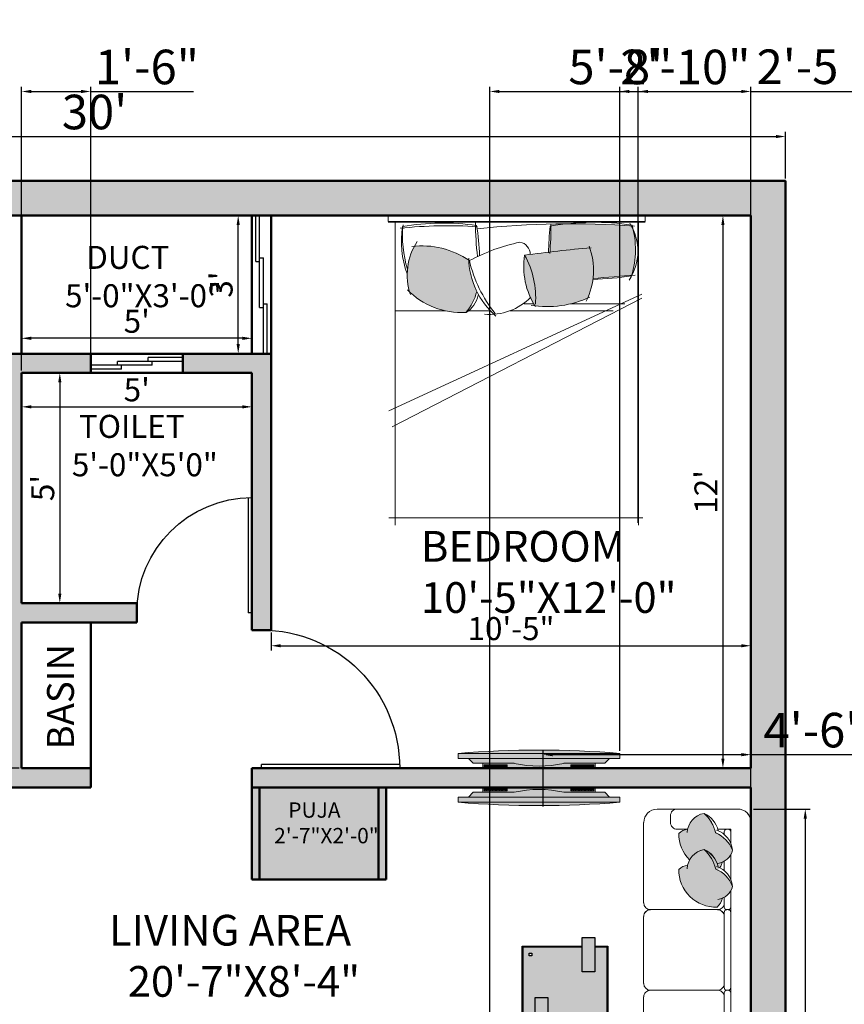
# Model space of a CAD drawing. Units: inches. Extents: x 3274 to 5176, y 1085 to 2172.
# Tile 14 of 16: x 4518 to 4733, y 1319 to 1575. Entities that reach past the tile are written whole.
import ezdxf

# ---------------------------------------------------------------- set-up
doc = ezdxf.new("R2010")
doc.units = ezdxf.units.IN
for name, color, linetype, lineweight in [('0.10', 252, 'Continuous', 9), ('A-ANNO-DIMS', 2, 'Continuous', 18), ('A-AREA-IDEN', 3, 'Continuous', 25), ('A-DOOR', 4, 'Continuous', 25), ('A-EQPM', 8, 'Continuous', 18), ('A-FLOR-PATT', 252, 'Continuous', 13), ('A-FURN', 8, 'Continuous', 18), ('A-GLAZ', 5, 'Continuous', 25), ('A-WALL', 7, 'Continuous', 50), ('A-WALL-PATT', 8, 'Continuous', 13), ('moveis', 254, 'Continuous', 5), ('parede', 7, 'Continuous', 30)]:
    doc.layers.add(name, color=color, linetype=linetype, lineweight=lineweight)
doc.layers.add('MOBIL', color=7, linetype='Continuous')
doc.styles.get("Standard").update_dxf_attribs({"font": 'arial.ttf'})
doc.dimstyles.new('ISO-25', dxfattribs={"dimtxt": 9, "dimasz": 2.5, "dimexe": 1.25, "dimexo": 0.625, "dimtad": 1, "dimdec": 1, "dimlunit": 3, "dimtxsty": 'Standard', "dimcen": 2.5, "dimclrd": 4, "dimclre": 4, "dimclrt": 1, "dimadec": 0, "dimazin": 0, "dimtfac": 1, "dimtdec": 1, "dimtmove": 0, "dimatfit": 3, "dimfxl": 1, "dimarcsym": 0})

# ---------------------------------------------------------------- blocks, each defined once
blk = doc.blocks.new('2')
for p, q in [((0, 30), (0, 0)), ((1, 30), (1, 0)), ((0, 0), (1, 0))]:
    blk.add_line(p, q)
blk.add_arc((0, 0), 30, 0, 90)
blk = doc.blocks.new('1')
for p, q in [((0, 36), (0, 0)), ((1, 36), (1, 0)), ((0, 0), (1, 0))]:
    blk.add_line(p, q)
blk.add_arc((0, 0), 36, 0, 90)
blk = doc.blocks.new('*D6')
at = {"layer": 'A-ANNO-DIMS', "color": 0, "lineweight": -2, "transparency": 16777216}
for p, q in [((4357.19, 1533.98), (4357.19, 1546.17)), ((4359.69, 1544.92), (4714.69, 1544.92)), ((4717.19, 1533.98), (4717.19, 1546.17))]:
    blk.add_line(p, q, dxfattribs=at)
at = {"layer": 'A-ANNO-DIMS', "color": 0, "transparency": 16777216}
for points in [[(4359.69, 1545.33), (4359.69, 1544.5), (4357.19, 1544.92)], [(4714.69, 1545.33), (4714.69, 1544.5), (4717.19, 1544.92)]]:
    blk.add_solid(points, dxfattribs=at)
at = {"layer": 'Defpoints', "color": 0, "transparency": 16777216}
for p in [(4717.19, 1544.92), (4357.19, 1533.35), (4717.19, 1533.35)]:
    blk.add_point(p, dxfattribs=at)
at = {"layer": 'A-ANNO-DIMS', "color": 0, "transparency": 16777216, "insert": (4537.19, 1550.14), "char_height": 9, "attachment_point": 5}
blk.add_mtext("30'", dxfattribs=at)
blk = doc.blocks.new('camita')
at = {"layer": '0.10'}
for p, q in [((-0.85, -0.045), (0.85, -0.045)), ((-0.805, -0.045), (-0.805, -2.0485)), ((0.805, -0.045), (0.805, -2.0485)), ((-0.8271, -0.521), (0.8464, -1.2932)), ((-0.8271, -0.5476), (0.8236, -1.3992)), ((-0.7161, -0.585), (-0.3554, -0.585)), ((-0.1136, -0.585), (-0.0485, -0.585)), ((-0.638, -0.63), (0.0434, -0.63)), ((0.1749, -0.63), (0.3179, -0.63)), ((0.4739, -0.63), (0.805, -0.63)), ((-0.8354, -2), (0.8464, -2))]:
    blk.add_line(p, q, dxfattribs=at)
blk.add_lwpolyline([(-0.85, -0.0405), (0.85, -0.0405), (0.85, 0), (-0.85, 0)], close=True, dxfattribs=at)
for centre, radius, start, end in [((-0.4574, -0.2364), 0.3443, 147.50996, 213.83359), ((-0.1997, -0.2266), 0.5864, 163.92635, 197.14087), ((-0.3639, -5.8457), 5.7909, 83.80731, 94.12107), ((-0.5104, -1.7232), 1.6781, 80.12554, 98.66187), ((2.3534, -0.0532), 2.5803, 180.10628, 184.38541), ((-1.4396, -0.0609), 1.7117, 352.92911, 0.39592), ((0.4863, -1.6286), 1.5781, 80.16015, 98.05996), ((0.0294, -0.1377), 0.7262, 342.58415, 6.00484), ((-1.5443, -0.2452), 1.3333, 359.93941, 7.55329), ((1.5815, -0.2893), 1.3353, 170.38021, 178.99138), ((0.4524, -3.0675), 2.9996, 83.90257, 93.67595), ((0.1326, -0.1696), 0.6307, 339.92303, 8.74334), ((-0.007, -0.258), 0.0828, 100.01798, 179.73597), ((-0.2931, -1.4378), 1.2903, 61.97485, 77.84351), ((0.3203, -0.3944), 0.4043, 341.45245, 33.45121), ((-0.0543, -0.3633), 0.4542, 159.30257, 206.50263), ((-1.3301, -9.6748), 9.4985, 82.27078, 84.93989), ((0.6265, -0.7518), 0.5508, 82.96906, 124.67388), ((0.4585, -0.5454), 0.5842, 151.04555, 184.14969), ((-0.5341, -0.3393), 0.4875, 327.26442, 9.0473), ((-0.1986, -0.2742), 0.5159, 310.73945, 359.05759), ((-0.5673, -0.0868), 0.9057, 321.69527, 346.46261), ((-1.8672, -14.986), 14.6323, 84.65974, 85.75157), ((-0.4598, 1.4861), 1.9092, 260.95299, 268.65169), ((0.5707, -0.4317), 0.3145, 192.93877, 221.96363), ((0.3612, -0.133), 0.5096, 267.25889, 315.29965), ((-0.2002, 0.064), 0.6673, 244.78094, 279.06058), ((0.179, -0.272), 0.3828, 224.52836, 275.22287), ((0.4384, -0.4834), 0.1898, 193.68485, 236.70352)]:
    blk.add_arc(centre, radius, start, end, dxfattribs=at)
blk = doc.blocks.new('SOFA 1')
at = {"transparency": 33554687}
h = blk.add_hatch(color=256, dxfattribs=at)
h.dxf.hatch_style = 1
h.paths.add_polyline_path([(3769.65, 1307.6, 0.084911), (3767.15, 1309.12, 0.046133), (3766.46, 1311.13), (3759.18, 1311.13, 0.039409), (3758.92, 1310.24, 0.165523), (3756.31, 1309.02, 0.42585), (3767.59, 1297.95, 0.121928), (3769.15, 1300.58, 0.027403), (3769.65, 1300.83)])
h.paths.add_polyline_path([(3765.34, 1313.08), (3760.4, 1313.08, 0.097704), (3759.18, 1311.13), (3766.46, 1311.13, 0.04873)])
h.paths.add_polyline_path([(3763.76, 1314.88, 0.16488), (3760.4, 1313.08), (3765.34, 1313.08, 0.051917)])
h.paths.add_polyline_path([(3771.6, 1305.17, 0.090388), (3769.65, 1307.6), (3769.65, 1300.83, 0.136035), (3771.6, 1302.77)])
h = blk.add_hatch(color=256, dxfattribs=at)
h.dxf.hatch_style = 1
h.paths.add_polyline_path([(3723.52, 1308.63, 0.147724), (3717.76, 1305.24, 0.310469), (3722.42, 1300.4), (3722.42, 1300.25, 0.156703), (3723.62, 1297.8, 0.425821), (3734.69, 1309.08, 0.121928), (3732.05, 1310.63, 0.233216), (3728.6, 1313.59, 0.213835)])
h = blk.add_hatch(color=256, dxfattribs=at)
h.dxf.hatch_style = 1
h.paths.add_polyline_path([(3769.16, 1235.96, 0.122267), (3767.6, 1238.61, 0.425972), (3756.32, 1227.54, 0.165563), (3758.93, 1226.32, 0.309481), (3763.76, 1221.69, 0.002677), (3763.83, 1221.72, 0.146094), (3767.16, 1227.43, 0.212433), (3772.1, 1232.48, 0.235342)])
h = blk.add_hatch(color=256, dxfattribs=at)
h.dxf.hatch_style = 1
h.paths.add_polyline_path([(3769.16, 1225.36, 0.122267), (3767.6, 1228.01, 0.425972), (3756.32, 1216.94, 0.165563), (3758.93, 1215.72, 0.309481), (3763.76, 1211.09, 0.002677), (3763.83, 1211.12, 0.146094), (3767.16, 1216.83, 0.212433), (3772.1, 1221.88, 0.235342)])
for p, q in [((3720.45, 1316.13), (3773.58, 1316.13)), ((3777.51, 1312.19), (3777.51, 1213.72))]:
    blk.add_line(p, q, dxfattribs=at)
for points in [[(3763.76, 1314.88, -0.147724), (3767.15, 1309.12, -0.213355), (3772.1, 1304.05, 0.213355), (3767.15, 1309.12, 0.147724), (3763.76, 1314.88, -0.249545), (3767.86, 1309.77, 0.249545), (3763.77, 1314.89, 0.356779), (3758.8, 1309.23, -0.356779), (3763.76, 1314.88)], [(3717.76, 1305.24, -0.147724), (3723.52, 1308.63, -0.213355), (3728.59, 1313.59, 0.213355), (3723.52, 1308.63, 0.147724), (3717.76, 1305.24, -0.249545), (3722.86, 1309.34, 0.249545), (3717.75, 1305.25, 0.356779), (3723.4, 1300.28, -0.356779), (3717.76, 1305.24)], [(3728.58, 1313.6, -0.306333), (3732.42, 1309.31, 0.306333), (3728.58, 1313.6, 0.306674), (3722.72, 1308.89, -0.306674), (3728.58, 1313.6)], [(3734.69, 1309.08, -0.425972), (3723.62, 1297.8, -0.165552), (3722.4, 1300.4, 0.165552), (3723.62, 1297.79, 0.425972), (3734.69, 1309.07, 0.121514), (3732.07, 1310.63, -0.121514), (3734.69, 1309.08)], [(3767.6, 1297.95, -0.425972), (3756.31, 1309.01, -0.165552), (3758.92, 1310.24, 0.165552), (3756.31, 1309.02, 0.425972), (3767.59, 1297.95, 0.121514), (3769.14, 1300.57, -0.121514), (3767.6, 1297.95)], [(3772.11, 1304.06, -0.306333), (3767.83, 1300.22, 0.306333), (3772.11, 1304.06, 0.306674), (3767.4, 1309.91, -0.306674), (3772.11, 1304.06)], [(3770.44, 1286.63, -0.414214), (3769.66, 1287.4, 0.414214), (3770.44, 1286.63, 0.414214), (3769.66, 1285.83, -0.414214), (3770.44, 1286.63)], [(3748.01, 1262.99, -0.414214), (3746.05, 1264.95, 0.414214), (3748.01, 1262.97, 0.414213), (3746.05, 1261.01, -0.414213), (3748.01, 1262.99)], [(3770.44, 1262.99, -0.414214), (3769.66, 1263.77, 0.414214), (3770.44, 1262.99, 0.414214), (3769.66, 1262.19, -0.414214), (3770.44, 1262.99)], [(3770.83, 1262.97, -0.414214), (3771.61, 1262.19, 0.414214), (3770.83, 1262.99, 0.414214), (3771.61, 1263.77, -0.414214), (3770.83, 1262.97)], [(3748.01, 1239.35, -0.414214), (3746.05, 1241.31, 0.414214), (3748.01, 1239.33, 0.414213), (3746.05, 1237.37, -0.414213), (3748.01, 1239.35)], [(3767.7, 1239.33, -0.414214), (3769.66, 1237.37, 0.414214), (3767.7, 1239.35, 0.414214), (3769.66, 1241.31, -0.414214), (3767.7, 1239.33)], [(3770.44, 1239.35, -0.414214), (3769.66, 1240.13, 0.414214), (3770.44, 1239.33, 0.414214), (3769.66, 1238.55, -0.414214), (3770.44, 1239.35)], [(3770.83, 1239.33, -0.414214), (3771.61, 1238.55, 0.414214), (3770.83, 1239.35, 0.414214), (3771.61, 1240.13, -0.414214), (3770.83, 1239.33)], [(3756.32, 1227.54, -0.425972), (3767.6, 1238.61, -0.121514), (3769.16, 1235.98, 0.121514), (3767.6, 1238.61, 0.425972), (3756.32, 1227.54, 0.165552), (3758.93, 1226.32, -0.165552), (3756.32, 1227.54)], [(3772.1, 1232.5, -0.306674), (3767.41, 1226.64, 0.306674), (3772.1, 1232.5, 0.306333), (3767.84, 1236.34, -0.306333), (3772.1, 1232.5)], [(3763.78, 1221.67, 0.249545), (3767.87, 1226.78, -0.249545), (3763.76, 1221.69, -0.356779), (3758.81, 1227.32, 0.356779), (3763.77, 1221.68, 0.147724), (3767.16, 1227.43, 0.213355), (3772.11, 1232.51, -0.213355), (3767.16, 1227.43, -0.147724), (3763.78, 1221.67)], [(3756.32, 1216.94, -0.200233), (3759.49, 1224.76, 0.200233), (3756.32, 1216.94, 0.165552), (3758.93, 1215.72, -0.165552), (3756.32, 1216.94)], [(3772.1, 1221.9, -0.306674), (3767.41, 1216.04, 0.306674), (3772.1, 1221.9, -0.213355), (3767.16, 1216.83, -0.147724), (3763.77, 1211.08, 0.147724), (3767.15, 1216.83, 0.213355), (3772.1, 1221.9)], [(3763.76, 1211.09, -0.356779), (3758.81, 1216.72, 0.356779), (3763.76, 1211.09, 0.249545), (3767.87, 1216.18, -0.249545), (3763.76, 1211.09)]]:
    blk.add_lwpolyline(points, format="xyb", dxfattribs=at)
for points in [[(3716.51, 1312.2), (3716.51, 1291.44)], [(3722.42, 1313.08), (3722.42, 1309.23), (3722.42, 1313.08), (3726.57, 1313.08)], [(3729.85, 1313.08), (3745.25, 1313.08)], [(3746.01, 1312.3), (3746.01, 1288.55)], [(3768.11, 1313.08), (3746.78, 1313.08)], [(3771.6, 1313.08), (3767.75, 1313.08), (3771.6, 1313.08), (3771.6, 1308.93)], [(3769.66, 1287.39), (3769.65, 1312.3)], [(3771.6, 1313.08), (3771.61, 1233.74)], [(3723.21, 1311.13), (3723.93, 1311.13)], [(3731.82, 1311.13), (3745.25, 1311.13)], [(3746.01, 1310.97), (3746.01, 1311.36)], [(3768.87, 1311.13), (3746.78, 1311.13)], [(3769.65, 1309.43), (3769.65, 1308.71)], [(3746.01, 1288.54), (3746.01, 1308.23)], [(3722.42, 1300.39), (3722.42, 1297.33)], [(3720.45, 1295.38), (3718.48, 1295.38)], [(3720.45, 1287.5), (3744.09, 1287.5)], [(3747.99, 1286.6), (3767.69, 1286.6)], [(3746.02, 1284.63), (3746.02, 1264.94)], [(3769.66, 1263.75), (3769.66, 1285.81)], [(3769.66, 1277.18), (3769.66, 1263.75)], [(3747.99, 1262.97), (3767.69, 1262.97)], [(3770.43, 1262.97), (3770.82, 1262.97)], [(3746.02, 1260.99), (3746.02, 1241.3)], [(3769.66, 1240.12), (3769.66, 1262.18)], [(3746.02, 1237.36), (3746.02, 1213.74)], [(3747.99, 1239.33), (3767.69, 1239.33)], [(3769.66, 1235.71), (3769.66, 1238.54)], [(3770.43, 1239.33), (3770.82, 1239.33)], [(3771.61, 1223.14), (3771.61, 1230.47)], [(3769.66, 1225.11), (3769.66, 1227.82)], [(3767.76, 1215.72), (3771.61, 1215.72), (3771.61, 1219.84), (3771.61, 1215.72)], [(3769.66, 1216.5), (3769.66, 1217.22)], [(3753.91, 1211.77), (3753.91, 1213.74)], [(3755.86, 1215.72), (3758.92, 1215.72)], [(3749.97, 1209.8), (3773.58, 1209.8)]]:
    blk.add_lwpolyline(points, close=True, dxfattribs=at)
for points in [[(3722.42, 1311.91, 0.414214), (3723.2, 1311.13, -0.414214)], [(3770.43, 1313.08, 0.414214), (3769.65, 1312.3, -0.414214)], [(3771.6, 1312.3, 0.414214), (3770.82, 1313.08, -0.414214)], [(3716.51, 1297.34, 0.414214), (3718.47, 1295.38, -0.414214)], [(3720.44, 1295.38, 0.414214), (3722.4, 1297.34, -0.414214)], [(3716.51, 1291.45, 0.414212), (3720.44, 1287.52, -0.414212)], [(3746.03, 1288.56, 0.414214), (3747.99, 1286.6, 0.414213), (3746.03, 1284.64, -0.414213), (3747.99, 1286.6, -0.414214)], [(3769.66, 1284.64, 0.414214), (3767.7, 1286.6, 0.414214), (3769.66, 1288.56, -0.414214), (3767.7, 1286.6, -0.414214)], [(3769.66, 1261.01, 0.414214), (3767.7, 1262.97, 0.414214), (3769.66, 1264.93, -0.414214), (3767.7, 1262.97, -0.414214)], [(3772.13, 1221.9, 0.306333), (3767.84, 1225.74, -0.306333)], [(3769.16, 1225.36, 0.071861), (3768.39, 1227.01, -0.071861)], [(3746.05, 1213.76, 0.414212), (3749.98, 1209.82, -0.414212)], [(3755.87, 1215.72, 0.414214), (3753.91, 1213.76, -0.414214)], [(3769.66, 1216.52, 0.414214), (3770.44, 1215.74, -0.414214)], [(3770.83, 1215.74, 0.414214), (3771.61, 1216.52, -0.414214)], [(3755.87, 1209.8, -0.414214), (3753.91, 1211.76, 0.414214)]]:
    blk.add_lwpolyline(points, format="xyb", close=True, dxfattribs=at)
for centre, radius, start, end in [((3720.44, 1312.2), 3.93, 90.0002, 179.9998), ((3720.44, 1312.19), 3.94, 89.9158, 179.9154), ((3773.58, 1312.2), 3.93, 0.0002, 89.9998), ((3773.57, 1312.19), 3.94, 359.9158, 89.9154), ((3745.22, 1312.29), 0.789, 0.8425, 90.8425), ((3745.24, 1311.91), 0.777, 270, 0), ((3745.24, 1311.91), 0.777, 270, 0), ((3746.8, 1312.29), 0.789, 89.1575, 179.1575), ((3746.79, 1311.91), 0.777, 180, 270), ((3746.79, 1311.91), 0.777, 180, 270), ((3768.87, 1312.3), 0.777, 360, 90), ((3768.87, 1311.91), 0.777, 270, 0), ((3744.09, 1309.21), 1.92, 358.766, 90.5111), ((3747.93, 1309.21), 1.92, 89.4889, 181.234), ((3744.08, 1289.48), 1.96, 270, 360), ((3744.08, 1289.48), 1.96, 270, 360), ((3773.58, 1213.73), 3.93, 270.0002, 359.9998), ((3773.59, 1213.73), 3.93, 269.9156, 359.9152)]:
    blk.add_arc(centre, radius, start, end, dxfattribs=at)
blk = doc.blocks.new('Mesa de centro Cantria feeling')
at = {"layer": 'MOBIL', "ltscale": 0.2}
h = blk.add_hatch(color=256, dxfattribs=at)
h.set_gradient(color1=(74, 55, 38), color2=(104, 77, 54), one_color=1, tint=0.31, name='CYLINDER')
h.paths.add_polyline_path([(-0.85, -0.3), (-0.7, -0.3), (-0.7, 0.1), (-0.85, 0.1)])
h = blk.add_hatch(color=256, dxfattribs=at)
h.set_gradient(color1=(221, 221, 223), one_color=1, tint=1)
h.paths.add_polyline_path([(-0.15, -0.6), (-0.15, -0.89), (-0.01, -0.89), (-0.01, -0.01), (-0.7, -0.01), (-0.7, -0.3), (-0.85, -0.3), (-0.85, -0.01), (-0.99, -0.01), (-0.99, -0.89), (-0.3, -0.89), (-0.3, -0.6)])
h.paths.add_polyline_path([(-0.112, -0.112), (-0.112, -0.082), (-0.082, -0.082), (-0.082, -0.112)], flags=16)
h.paths.add_polyline_path([(-0.888, -0.788), (-0.888, -0.818), (-0.918, -0.818), (-0.918, -0.788)], flags=16)
h = blk.add_hatch(color=256, dxfattribs=at)
h.set_gradient(color1=(74, 55, 38), color2=(104, 77, 54), one_color=1, tint=0.31, name='CYLINDER')
h.paths.add_polyline_path([(-0.15, -0.6), (-0.3, -0.6), (-0.3, -1), (-0.15, -1)])
for points in [[(-0.85, 0), (-1, 0), (-1, -0.9), (-0.3, -0.9)], [(-0.15, -0.9), (0, -0.9), (0, 0), (-0.7, 0)], [(-0.85, -0.01), (-0.99, -0.01), (-0.99, -0.89), (-0.3, -0.89)], [(-0.15, -0.89), (-0.01, -0.89), (-0.01, -0.01), (-0.7, -0.01)]]:
    blk.add_lwpolyline(points, dxfattribs=at)
for points in [[(-0.85, -0.3), (-0.7, -0.3), (-0.7, 0.1), (-0.85, 0.1)], [(-0.082, -0.082), (-0.112, -0.082), (-0.112, -0.112), (-0.082, -0.112)], [(-0.15, -0.6), (-0.3, -0.6), (-0.3, -1), (-0.15, -1)], [(-0.918, -0.818), (-0.888, -0.818), (-0.888, -0.788), (-0.918, -0.788)]]:
    blk.add_lwpolyline(points, close=True, dxfattribs=at)
blk = doc.blocks.new('PLASMA 2')
at = {"layer": 'moveis', "ltscale": 0.08}
h = blk.add_hatch(dxfattribs=at)
h.set_pattern_fill('_USER,_O', color=256, scale=0.008, double=1, pattern_type=0)
h.set_pattern_definition([(360, (-4.134502, -6.848382), (0, 0.008), []), (90, (-4.134502, -6.848382), (-0.008, 0), [])])
h.paths.add_polyline_path([(-0.2099, -0.0965), (-0.3623, -0.0965), (-0.3623, -0.1111), (-0.2099, -0.1111)])
h = blk.add_hatch(dxfattribs=at)
h.set_pattern_fill('_USER,_O', color=256, scale=0.008, double=1, pattern_type=0)
h.set_pattern_definition([(180, (4.134502, -6.848382), (0, 0.008), []), (90, (4.134502, -6.848382), (0.008, 0), [])])
h.paths.add_polyline_path([(0.2099, -0.0965), (0.3623, -0.0965), (0.3623, -0.1111), (0.2099, -0.1111)])
at = {"layer": 'parede', "ltscale": 0.08}
h = blk.add_hatch(color=256, dxfattribs=at)
h.dxf.hatch_style = 1
h.set_gradient(color1=(131, 136, 145), one_color=1, tint=1, name='CURVED')
h.paths.add_polyline_path([(-0.535, -0.0215), (0.535, -0.0215, 0.040195)])
h = blk.add_hatch(color=256, dxfattribs=at)
h.dxf.hatch_style = 1
h.set_gradient(color1=(131, 136, 145), color2=(0, 0, 0), one_color=1, name='CURVED')
h.paths.add_polyline_path([(0.535, -0.0215), (-0.535, -0.0215), (-0.535, -0.0553), (0.535, -0.0553)])
h = blk.add_hatch(color=256, dxfattribs=at)
h.dxf.hatch_style = 1
h.set_gradient(color1=(131, 136, 145), one_color=1, tint=1, name='CYLINDER')
h.paths.add_polyline_path([(0.4673, -0.0553), (-0.4673, -0.0553), (-0.4363, -0.0876), (-0.1636, -0.0876, 0.114423), (0.1636, -0.0876), (0.4363, -0.0876)])
h = blk.add_hatch(color=256, dxfattribs=at)
h.dxf.hatch_style = 1
h.set_gradient(color1=(131, 136, 145), color2=(0, 0, 0), one_color=1, name='CURVED')
h.paths.add_polyline_path([(0.3724, -0.0876), (0.1636, -0.0876, -0.114423), (-0.1636, -0.0876), (-0.3724, -0.0876), (-0.3724, -0.12), (0.3724, -0.12)])
h.paths.add_polyline_path([(-0.2099, -0.1111), (-0.3623, -0.1111), (-0.3623, -0.0965), (-0.2099, -0.0965)], flags=16)
h.paths.add_polyline_path([(0.2099, -0.1111), (0.2099, -0.0965), (0.3623, -0.0965), (0.3623, -0.1111)], flags=16)
at = {"layer": 'moveis', "ltscale": 0.08}
for p, q in [((-0.535, -0.0215), (-0.535, -0.0553)), ((-0.535, -0.0215), (0.535, -0.0215)), ((0.535, -0.0553), (-0.535, -0.0553)), ((-0.4673, -0.0553), (-0.4363, -0.0876)), ((0.4673, -0.0553), (0.4363, -0.0876)), ((0.535, -0.0553), (0.535, -0.0215)), ((-0.4363, -0.0876), (-0.1636, -0.0876)), ((-0.3724, -0.0876), (-0.3724, -0.12)), ((-0.3724, -0.12), (0.3724, -0.12)), ((0.1636, -0.0876), (0.4363, -0.0876)), ((0.3724, -0.0876), (0.3724, -0.12))]:
    blk.add_line(p, q, dxfattribs=at)
for points in [[(-0.3623, -0.0965), (-0.2099, -0.0965), (-0.2099, -0.1111), (-0.3623, -0.1111)], [(0.3623, -0.0965), (0.2099, -0.0965), (0.2099, -0.1111), (0.3623, -0.1111)]]:
    blk.add_lwpolyline(points, close=True, dxfattribs=at)
for centre, radius, start, end in [((0, -6.6658), 6.6658, 85.39647, 94.60353), ((0, 0.6178), 0.7242, 256.94486, 283.05514)]:
    blk.add_arc(centre, radius, start, end, dxfattribs=at)
blk = doc.blocks.new('*D70')
at = {"layer": 'A-ANNO-DIMS', "color": 0, "lineweight": -2, "transparency": 16777216}
for p, q in [((4512.56, 1524.35), (4499.67, 1524.35)), ((4500.92, 1521.85), (4500.92, 1382.85)), ((4517.56, 1380.35), (4499.67, 1380.35))]:
    blk.add_line(p, q, dxfattribs=at)
at = {"layer": 'A-ANNO-DIMS', "color": 0, "transparency": 16777216}
for points in [[(4500.51, 1521.85), (4501.34, 1521.85), (4500.92, 1524.35)], [(4500.51, 1382.85), (4501.34, 1382.85), (4500.92, 1380.35)]]:
    blk.add_solid(points, dxfattribs=at)
at = {"layer": 'Defpoints', "color": 0, "transparency": 16777216}
for p in [(4513.19, 1524.35), (4500.92, 1380.35), (4518.19, 1380.35)]:
    blk.add_point(p, dxfattribs=at)
at = {"layer": 'A-ANNO-DIMS', "color": 0, "transparency": 16777216, "insert": (4497.29, 1452.35), "char_height": 6, "attachment_point": 5, "rotation": 90}
blk.add_mtext("12'", dxfattribs=at)
blk = doc.blocks.new('*D83')
at = {"layer": 'A-ANNO-DIMS', "color": 0, "lineweight": -2, "transparency": 16777216}
for p, q in [((4518.19, 1482.73), (4518.19, 1473.25)), ((4578.19, 1482.73), (4578.19, 1473.25)), ((4520.69, 1474.5), (4575.69, 1474.5))]:
    blk.add_line(p, q, dxfattribs=at)
at = {"layer": 'A-ANNO-DIMS', "color": 0, "transparency": 16777216}
for points in [[(4520.69, 1474.91), (4520.69, 1474.08), (4518.19, 1474.5)], [(4575.69, 1474.91), (4575.69, 1474.08), (4578.19, 1474.5)]]:
    blk.add_solid(points, dxfattribs=at)
at = {"layer": 'Defpoints', "color": 0, "transparency": 16777216}
for p in [(4518.19, 1483.35), (4578.19, 1483.35), (4578.19, 1474.5)]:
    blk.add_point(p, dxfattribs=at)
at = {"layer": 'A-ANNO-DIMS', "color": 0, "transparency": 16777216, "insert": (4548.19, 1478.17), "char_height": 6, "attachment_point": 5}
blk.add_mtext("5'", dxfattribs=at)
blk = doc.blocks.new('*D84')
at = {"layer": 'A-ANNO-DIMS', "color": 0, "lineweight": -2, "transparency": 16777216}
for p, q in [((4518.81, 1483.35), (4529.39, 1483.35)), ((4528.14, 1480.85), (4528.14, 1425.85)), ((4518.81, 1423.35), (4529.39, 1423.35))]:
    blk.add_line(p, q, dxfattribs=at)
at = {"layer": 'A-ANNO-DIMS', "color": 0, "transparency": 16777216}
for points in [[(4527.72, 1480.85), (4528.55, 1480.85), (4528.14, 1483.35)], [(4527.72, 1425.85), (4528.55, 1425.85), (4528.14, 1423.35)]]:
    blk.add_solid(points, dxfattribs=at)
at = {"layer": 'Defpoints', "color": 0, "transparency": 16777216}
for p in [(4518.19, 1483.35), (4518.19, 1423.35), (4528.14, 1423.35)]:
    blk.add_point(p, dxfattribs=at)
at = {"layer": 'A-ANNO-DIMS', "color": 0, "transparency": 16777216, "insert": (4524.46, 1453.35), "char_height": 6, "attachment_point": 5, "rotation": 90}
blk.add_mtext("5'", dxfattribs=at)
blk = doc.blocks.new('*D85')
at = {"layer": 'A-ANNO-DIMS', "color": 0, "lineweight": -2, "transparency": 16777216}
for p, q in [((4518.19, 1488.98), (4518.19, 1493.6)), ((4578.19, 1488.98), (4578.19, 1493.6)), ((4575.69, 1492.35), (4520.69, 1492.35))]:
    blk.add_line(p, q, dxfattribs=at)
at = {"layer": 'A-ANNO-DIMS', "color": 0, "transparency": 16777216}
for points in [[(4520.69, 1492.77), (4520.69, 1491.93), (4518.19, 1492.35)], [(4575.69, 1492.77), (4575.69, 1491.93), (4578.19, 1492.35)]]:
    blk.add_solid(points, dxfattribs=at)
at = {"layer": 'Defpoints', "color": 0, "transparency": 16777216}
for p in [(4518.19, 1492.35), (4518.19, 1488.35), (4578.19, 1488.35)]:
    blk.add_point(p, dxfattribs=at)
at = {"layer": 'A-ANNO-DIMS', "color": 0, "transparency": 16777216, "insert": (4548.19, 1496.02), "char_height": 6, "attachment_point": 5}
blk.add_mtext("5'", dxfattribs=at)
blk = doc.blocks.new('*D86')
at = {"layer": 'A-ANNO-DIMS', "color": 0, "lineweight": -2, "transparency": 16777216}
for p, q in [((4577.56, 1524.35), (4573.37, 1524.35)), ((4574.62, 1490.85), (4574.62, 1521.85)), ((4577.56, 1488.35), (4573.37, 1488.35))]:
    blk.add_line(p, q, dxfattribs=at)
at = {"layer": 'A-ANNO-DIMS', "color": 0, "transparency": 16777216}
for points in [[(4574.2, 1521.85), (4575.03, 1521.85), (4574.62, 1524.35)], [(4574.2, 1490.85), (4575.03, 1490.85), (4574.62, 1488.35)]]:
    blk.add_solid(points, dxfattribs=at)
at = {"layer": 'Defpoints', "color": 0, "transparency": 16777216}
for p in [(4574.62, 1524.35), (4578.19, 1524.35), (4578.19, 1488.35)]:
    blk.add_point(p, dxfattribs=at)
at = {"layer": 'A-ANNO-DIMS', "color": 0, "transparency": 16777216, "insert": (4570.93, 1506.35), "char_height": 6, "attachment_point": 5, "rotation": 90}
blk.add_mtext("3'", dxfattribs=at)
blk = doc.blocks.new('*D87')
at = {"layer": 'A-ANNO-DIMS', "color": 0, "lineweight": -2, "transparency": 16777216}
for p, q in [((4707.56, 1524.35), (4699.65, 1524.35)), ((4700.9, 1521.85), (4700.9, 1382.85)), ((4707.56, 1380.35), (4699.65, 1380.35))]:
    blk.add_line(p, q, dxfattribs=at)
at = {"layer": 'A-ANNO-DIMS', "color": 0, "transparency": 16777216}
for points in [[(4700.48, 1521.85), (4701.31, 1521.85), (4700.9, 1524.35)], [(4700.48, 1382.85), (4701.31, 1382.85), (4700.9, 1380.35)]]:
    blk.add_solid(points, dxfattribs=at)
at = {"layer": 'Defpoints', "color": 0, "transparency": 16777216}
for p in [(4708.19, 1524.35), (4700.9, 1380.35), (4708.19, 1380.35)]:
    blk.add_point(p, dxfattribs=at)
at = {"layer": 'A-ANNO-DIMS', "color": 0, "transparency": 16777216, "insert": (4697.26, 1452.35), "char_height": 6, "attachment_point": 5, "rotation": 90}
blk.add_mtext("12'", dxfattribs=at)
blk = doc.blocks.new('*D88')
at = {"layer": 'A-ANNO-DIMS', "color": 0, "lineweight": -2, "transparency": 16777216}
for p, q in [((4583.19, 1415.73), (4583.19, 1411.01)), ((4708.19, 1415.73), (4708.19, 1411.01)), ((4585.69, 1412.26), (4705.69, 1412.26))]:
    blk.add_line(p, q, dxfattribs=at)
at = {"layer": 'A-ANNO-DIMS', "color": 0, "transparency": 16777216}
for points in [[(4585.69, 1412.68), (4585.69, 1411.85), (4583.19, 1412.26)], [(4705.69, 1412.68), (4705.69, 1411.85), (4708.19, 1412.26)]]:
    blk.add_solid(points, dxfattribs=at)
at = {"layer": 'Defpoints', "color": 0, "transparency": 16777216}
for p in [(4583.19, 1416.35), (4708.19, 1416.35), (4708.19, 1412.26)]:
    blk.add_point(p, dxfattribs=at)
at = {"layer": 'A-ANNO-DIMS', "color": 0, "transparency": 16777216, "insert": (4645.69, 1415.95), "char_height": 6, "attachment_point": 5}
blk.add_mtext('10\'-5"', dxfattribs=at)
blk = doc.blocks.new('WIN-24')
for p, q in [((4552.19, 1485.35), (4536.19, 1485.35)), ((4560.19, 1486.35), (4543.19, 1486.35)), ((4543.19, 1485.35), (4543.19, 1486.35)), ((4544.19, 1484.35), (4544.19, 1485.35)), ((4551.19, 1486.35), (4551.19, 1487.35)), ((4560.19, 1487.35), (4551.19, 1487.35)), ((4552.19, 1485.35), (4552.19, 1486.35)), ((4544.19, 1484.35), (4536.19, 1484.35))]:
    blk.add_line(p, q)
blk = doc.blocks.new('WIN-36')
for p, q in [((4514.19, 1512.35), (4514.19, 1524.35)), ((4515.19, 1500.35), (4515.19, 1524.35)), ((4515.19, 1513.35), (4516.19, 1513.35)), ((4516.19, 1488.35), (4516.19, 1513.35)), ((4514.19, 1512.35), (4515.19, 1512.35)), ((4516.19, 1501.35), (4517.19, 1501.35)), ((4517.19, 1488.35), (4517.19, 1501.35)), ((4515.19, 1500.35), (4516.19, 1500.35))]:
    blk.add_line(p, q)
blk = doc.blocks.new('*D136')
at = {"layer": 'A-ANNO-DIMS', "color": 4, "lineweight": -2, "transparency": 16777216}
for p, q in [((4708.83, 1369.73), (4723.61, 1369.73)), ((4722.36, 1367.23), (4722.36, 1277.84)), ((4708.83, 1275.34), (4723.61, 1275.34)), ((4722.36, 1275.34), (4722.36, 1085.06))]:
    blk.add_line(p, q, dxfattribs=at)
at = {"layer": 'A-ANNO-DIMS', "color": 4, "transparency": 16777216}
for points in [[(4721.94, 1367.23), (4722.78, 1367.23), (4722.36, 1369.73)], [(4721.94, 1277.84), (4722.78, 1277.84), (4722.36, 1275.34)]]:
    blk.add_solid(points, dxfattribs=at)
at = {"layer": 'Defpoints', "color": 0, "transparency": 16777216}
for p in [(4708.2, 1369.73), (4708.2, 1275.34), (4722.36, 1275.34)]:
    blk.add_point(p, dxfattribs=at)
at = {"layer": 'A-ANNO-DIMS', "color": 1, "transparency": 16777216, "insert": (4717.08, 1178.95), "char_height": 9, "attachment_point": 5, "rotation": 90}
blk.add_mtext('L-SHAPED SOFA 7\'-10 1/2" TYP.', dxfattribs=at)
blk = doc.blocks.new('*D137')
at = {"layer": 'A-ANNO-DIMS', "color": 4, "lineweight": -2, "transparency": 16777216}
for p, q in [((4654.05, 1370.36), (4654.05, 1385.14)), ((4708.2, 1370.36), (4708.2, 1385.14)), ((4656.55, 1383.89), (4705.7, 1383.89)), ((4708.2, 1383.89), (4767.17, 1383.89))]:
    blk.add_line(p, q, dxfattribs=at)
at = {"layer": 'A-ANNO-DIMS', "color": 4, "transparency": 16777216}
for points in [[(4656.55, 1384.31), (4656.55, 1383.47), (4654.05, 1383.89)], [(4705.7, 1384.31), (4705.7, 1383.47), (4708.2, 1383.89)]]:
    blk.add_solid(points, dxfattribs=at)
at = {"layer": 'Defpoints', "color": 0, "transparency": 16777216}
for p in [(4708.2, 1383.89), (4654.05, 1369.73), (4708.2, 1369.73)]:
    blk.add_point(p, dxfattribs=at)
at = {"layer": 'A-ANNO-DIMS', "color": 1, "transparency": 16777216, "insert": (4738.94, 1389.11), "char_height": 9, "attachment_point": 5}
blk.add_mtext('4\'-6" TYP.', dxfattribs=at)
blk = doc.blocks.new('*D154')
at = {"layer": 'A-ANNO-DIMS', "color": 4, "lineweight": -2, "transparency": 16777216}
for p, q in [((4640.19, 1275.98), (4640.19, 1557.9)), ((4708.19, 1275.98), (4708.19, 1557.9)), ((4642.69, 1556.65), (4705.69, 1556.65))]:
    blk.add_line(p, q, dxfattribs=at)
at = {"layer": 'A-ANNO-DIMS', "color": 4, "transparency": 16777216}
for points in [[(4642.69, 1557.07), (4642.69, 1556.24), (4640.19, 1556.65)], [(4705.69, 1557.07), (4705.69, 1556.24), (4708.19, 1556.65)]]:
    blk.add_solid(points, dxfattribs=at)
at = {"layer": 'Defpoints', "color": 0, "transparency": 16777216}
for p in [(4708.19, 1556.65), (4640.19, 1275.35), (4708.19, 1275.35)]:
    blk.add_point(p, dxfattribs=at)
at = {"layer": 'A-ANNO-DIMS', "color": 1, "transparency": 16777216, "insert": (4674.19, 1561.87), "char_height": 9, "attachment_point": 5}
blk.add_mtext('5\'-8"', dxfattribs=at)
blk = doc.blocks.new('*D155')
at = {"layer": 'A-ANNO-DIMS', "color": 4, "lineweight": -2, "transparency": 16777216}
for p, q in [((4518.19, 1483.98), (4518.19, 1557.9)), ((4536.19, 1483.98), (4536.19, 1557.9)), ((4520.69, 1556.65), (4533.69, 1556.65)), ((4536.19, 1556.65), (4563.01, 1556.65))]:
    blk.add_line(p, q, dxfattribs=at)
at = {"layer": 'A-ANNO-DIMS', "color": 4, "transparency": 16777216}
for points in [[(4520.69, 1557.07), (4520.69, 1556.24), (4518.19, 1556.65)], [(4533.69, 1557.07), (4533.69, 1556.24), (4536.19, 1556.65)]]:
    blk.add_solid(points, dxfattribs=at)
at = {"layer": 'Defpoints', "color": 0, "transparency": 16777216}
for p in [(4536.19, 1556.65), (4518.19, 1483.35), (4536.19, 1483.35)]:
    blk.add_point(p, dxfattribs=at)
at = {"layer": 'A-ANNO-DIMS', "color": 1, "transparency": 16777216, "insert": (4550.85, 1561.87), "char_height": 9, "attachment_point": 5}
blk.add_mtext('1\'-6"', dxfattribs=at)
blk = doc.blocks.new('*D157')
at = {"layer": 'A-ANNO-DIMS', "color": 4, "lineweight": -2, "transparency": 16777216}
for p, q in [((4678.86, 1444.32), (4678.86, 1557.9)), ((4708.19, 1380.98), (4708.19, 1557.9)), ((4681.36, 1556.65), (4705.69, 1556.65)), ((4708.19, 1556.65), (4756.99, 1556.65))]:
    blk.add_line(p, q, dxfattribs=at)
at = {"layer": 'A-ANNO-DIMS', "color": 4, "transparency": 16777216}
for points in [[(4681.36, 1557.07), (4681.36, 1556.24), (4678.86, 1556.65)], [(4705.69, 1557.07), (4705.69, 1556.24), (4708.19, 1556.65)]]:
    blk.add_solid(points, dxfattribs=at)
at = {"layer": 'Defpoints', "color": 0, "transparency": 16777216}
for p in [(4708.19, 1556.65), (4678.86, 1443.7), (4708.19, 1380.35)]:
    blk.add_point(p, dxfattribs=at)
at = {"layer": 'A-ANNO-DIMS', "color": 1, "transparency": 16777216, "insert": (4733.84, 1561.93), "char_height": 9, "attachment_point": 5}
blk.add_mtext('2\'-5 1/2"', dxfattribs=at)
blk = doc.blocks.new('*D159')
at = {"layer": 'A-ANNO-DIMS', "color": 4, "lineweight": -2, "transparency": 16777216}
for p, q in [((4674.06, 1384.86), (4674.06, 1557.9)), ((4708.19, 1380.98), (4708.19, 1557.9)), ((4676.56, 1556.65), (4705.69, 1556.65))]:
    blk.add_line(p, q, dxfattribs=at)
at = {"layer": 'A-ANNO-DIMS', "color": 4, "transparency": 16777216}
for points in [[(4676.56, 1557.07), (4676.56, 1556.24), (4674.06, 1556.65)], [(4705.69, 1557.07), (4705.69, 1556.24), (4708.19, 1556.65)]]:
    blk.add_solid(points, dxfattribs=at)
at = {"layer": 'Defpoints', "color": 0, "transparency": 16777216}
for p in [(4708.19, 1556.65), (4674.06, 1384.23), (4708.19, 1380.35)]:
    blk.add_point(p, dxfattribs=at)
at = {"layer": 'A-ANNO-DIMS', "color": 1, "transparency": 16777216, "insert": (4691.12, 1561.87), "char_height": 9, "attachment_point": 5}
blk.add_mtext('2\'-10"', dxfattribs=at)

msp = doc.modelspace()

# ---------------------------------------------------------------- hatches: boundary and pattern name
at = {"layer": 'A-FLOR-PATT'}
h = msp.add_hatch(color=256, dxfattribs=at)
h.dxf.hatch_style = 1
h.paths.add_polyline_path([(4666.2, 1515.92, -0.113891), (4667.06, 1507.93, -0.004387), (4677.14, 1508.78, 0.142222), (4677.26, 1521.65, 0.023222), (4656.1, 1522.13, -0.017944), (4655.83, 1514.85, -0.006967)])
h.paths.add_polyline_path([(4620.52, 1516.35, 0.194952), (4619.24, 1504.46, 0.202559), (4633.91, 1499.07, 0.127326), (4636.77, 1504.58, -0.104045), (4634.7, 1512.68, 0.173835)])
h = msp.add_hatch(color=256, dxfattribs=at)
h.dxf.hatch_style = 1
h.paths.add_polyline_path([(4677.52, 1520.67, 0.020657), (4677.01, 1521.67, 0.01851), (4660.14, 1522.19, 0.015442), (4656.1, 1521.63, -0.016701), (4655.83, 1514.85, -0.006967), (4666.2, 1515.92, -0.113891), (4667.06, 1507.93, -0.004387), (4677.14, 1508.78, 0.131047)])
h.paths.add_polyline_path([(4666.2, 1515.92, 0.006967), (4655.83, 1514.85, 0.00444), (4649.24, 1514.01, 0.181694), (4651.94, 1500.78, 0.134508), (4665.68, 1502.84, 0.189536)])
h = msp.add_hatch(color=256, dxfattribs=at)
h.dxf.hatch_style = 1
h.paths.add_polyline_path([(4613.19, 1375.35), (4611.19, 1375.35), (4611.19, 1351.35), (4613.19, 1351.35)])
h.paths.add_polyline_path([(4580.19, 1375.35), (4578.19, 1375.35), (4578.19, 1351.35), (4580.19, 1351.35)])
h = msp.add_hatch(color=256, dxfattribs=at)
h.dxf.hatch_style = 1
h.paths.add_polyline_path([(4611.19, 1351.35), (4611.19, 1375.35), (4580.19, 1375.35), (4580.19, 1351.35)])
h.paths.add_polyline_path([(4582.83, 1358.6), (4610.81, 1358.6), (4610.81, 1373.52), (4582.83, 1373.52)], flags=24)
at = {"layer": 'A-WALL-PATT'}
h = msp.add_hatch(color=256, dxfattribs=at)
h.dxf.hatch_style = 1
h.paths.add_polyline_path([(4717.19, 1533.35), (4357.19, 1533.35), (4357.19, 1173.35), (4390.19, 1173.35), (4390.19, 1182.35), (4366.19, 1182.35), (4366.19, 1266.35), (4426.19, 1266.35), (4426.19, 1271.35), (4366.19, 1271.35), (4366.19, 1375.35), (4426.19, 1375.35), (4426.19, 1380.35), (4366.19, 1380.35), (4366.19, 1524.35), (4708.19, 1524.35), (4708.19, 1380.35), (4578.19, 1380.35), (4578.19, 1375.35), (4708.19, 1375.35), (4708.19, 1275.35), (4640.19, 1275.35), (4640.19, 1266.35), (4708.19, 1266.35), (4708.19, 1182.35), (4666.19, 1182.35), (4666.19, 1173.35), (4717.19, 1173.35)])
h.paths.add_polyline_path([(4461.19, 1375.35), (4477.19, 1375.35), (4477.19, 1380.35), (4456.19, 1380.35), (4456.19, 1319.35), (4401.19, 1319.35), (4401.19, 1339.35), (4396.19, 1339.35), (4396.19, 1314.35), (4456.19, 1314.35), (4456.19, 1266.35), (4477.19, 1266.35), (4477.19, 1271.35), (4461.19, 1271.35)], flags=17)
h.paths.add_polyline_path([(4518.19, 1483.35), (4536.19, 1483.35), (4536.19, 1488.35), (4513.19, 1488.35), (4513.19, 1375.35), (4536.19, 1375.35), (4536.19, 1380.35), (4518.19, 1380.35), (4518.19, 1418.35), (4548.19, 1418.35), (4548.19, 1423.35), (4518.19, 1423.35)], flags=17)
h.paths.add_polyline_path([(4583.19, 1488.35), (4560.19, 1488.35), (4560.19, 1483.35), (4578.19, 1483.35), (4578.19, 1416.35), (4583.19, 1416.35)], flags=17)
h.paths.add_polyline_path([(4518.19, 1266.35), (4523.19, 1266.35), (4523.19, 1275.35), (4513.19, 1275.35), (4513.19, 1182.35), (4462.19, 1182.35), (4462.19, 1173.35), (4518.19, 1173.35)], flags=17)
h.paths.add_polyline_path([(4580.19, 1275.35), (4571.19, 1275.35), (4571.19, 1270.85), (4571.19, 1266.35), (4580.19, 1266.35)], flags=17)
h.paths.add_polyline_path([(4594.19, 1182.35), (4578.19, 1182.35), (4578.19, 1173.35), (4594.19, 1173.35)], flags=17)
h.paths.add_polyline_path([(4573.24, 1316.29), (4647.44, 1316.29), (4647.44, 1346.14), (4573.24, 1346.14)], flags=25)
h.paths.add_polyline_path([(4529.43, 1453), (4568.61, 1453), (4568.61, 1475.39), (4529.43, 1475.39)], flags=25)
h.paths.add_polyline_path([(4619, 1443.76), (4687.39, 1443.76), (4687.39, 1473.61), (4619, 1473.61)], flags=25)
h.paths.add_polyline_path([(4527.67, 1497.04), (4569.64, 1497.04), (4569.64, 1519.43), (4527.67, 1519.43)], flags=25)
h.paths.add_polyline_path([(4407.08, 1443.76), (4475.47, 1443.76), (4475.47, 1473.61), (4407.08, 1473.61)], flags=25)

# ---------------------------------------------------------------- linework, layer by layer
at = {"layer": 'A-WALL'}
for p, q in [((4366.19, 1524.35), (4708.19, 1524.35)), ((4518.19, 1488.35), (4518.19, 1524.35)), ((4578.19, 1524.35), (4578.19, 1488.35)), ((4583.19, 1524.35), (4583.19, 1416.35)), ((4708.19, 1524.35), (4708.19, 1380.35)), ((4513.19, 1488.35), (4583.19, 1488.35)), ((4536.19, 1483.35), (4536.19, 1488.35)), ((4560.19, 1483.35), (4560.19, 1488.35)), ((4518.19, 1483.35), (4578.19, 1483.35)), ((4518.19, 1423.35), (4518.19, 1483.35)), ((4578.19, 1483.35), (4578.19, 1416.35)), ((4518.19, 1423.35), (4548.19, 1423.35)), ((4548.19, 1423.35), (4548.19, 1418.35)), ((4518.19, 1418.35), (4548.19, 1418.35)), ((4518.19, 1380.35), (4518.19, 1418.35)), ((4536.19, 1375.35), (4536.19, 1418.35)), ((4578.19, 1416.35), (4583.19, 1416.35)), ((4518.19, 1380.35), (4536.19, 1380.35)), ((4578.19, 1380.35), (4578.19, 1351.35)), ((4578.19, 1380.35), (4708.19, 1380.35)), ((4513.19, 1375.35), (4536.19, 1375.35)), ((4578.19, 1375.35), (4708.19, 1375.35)), ((4580.19, 1375.35), (4580.19, 1351.35)), ((4611.19, 1375.35), (4611.19, 1351.35)), ((4613.19, 1375.35), (4613.19, 1351.35)), ((4708.19, 1375.35), (4708.19, 1275.35)), ((4578.19, 1351.35), (4613.19, 1351.35))]:
    msp.add_line(p, q, dxfattribs=at)
msp.add_lwpolyline([(4518.19, 1173.35), (4357.19, 1173.35), (4357.19, 1533.35), (4717.19, 1533.35), (4717.19, 1173.35), (4578.19, 1173.35)], dxfattribs=at)

# ---------------------------------------------------------------- block references
at = {"layer": 'A-DOOR', "xscale": -1}
msp.add_blockref('2', (4578.19, 1420.85), dxfattribs=at)
at = {"layer": 'A-DOOR', "xscale": -1, "rotation": 270}
msp.add_blockref('1', (4580.69, 1380.35), dxfattribs=at)
at = {"layer": 'A-EQPM', "xscale": 39.37, "yscale": 39.37, "zscale": 39.37}
msp.add_blockref('PLASMA 2', (4652.99, 1385.08), dxfattribs=at)
at = {"layer": 'A-EQPM', "xscale": -39.37, "yscale": 39.37, "zscale": 39.37, "rotation": 180}
msp.add_blockref('PLASMA 2', (4652.99, 1370.63), dxfattribs=at)
at = {"layer": 'A-FURN', "xscale": -39.375, "yscale": 39.375, "zscale": 39.375}
msp.add_blockref('camita', (4647.17, 1524.35), dxfattribs=at)
at = {"layer": 'A-FURN', "rotation": 180}
for name, p, xscale, yscale, zscale in [('SOFA 1', (1355.08, 2443.61), -0.887653230693335, 0.887653230693335, 0.887653230693335), ('Mesa de centro Cantria feeling', (4670.91, 1313.94), -22.3138190187957, 22.3138190187957, 22.3138190187957)]:
    msp.add_blockref(name, p, dxfattribs=dict(at, xscale=xscale, yscale=yscale, zscale=zscale))
at = {"layer": 'A-GLAZ'}
for name, p in [('WIN-36', (65, 0)), ('WIN-24', (0, 0))]:
    msp.add_blockref(name, p, dxfattribs=at)

# ---------------------------------------------------------------- texts
at = {"layer": 'A-AREA-IDEN', "attachment_point": 1}
for s, width, heights, insert, char_height in [('   DUCT\\P5\'-0"X3\'-0"', 58.0121, [16.24], (4529.52, 1516.44), 6), (' TOILET\\P5\'-0"X5\'0"', 58.0121, [0], (4531.28, 1472.41), 6), ('BEDROOM\\P10\'-5"X12\'-0"', 58.0121, [0], (4622.22, 1442.16), 8), ('   PUJA\\P2\'-7"X2\'-0"', 58.0121, [16.24], (4583.99, 1371.46), 4), ('LIVING AREA\\P  20\'-7"X8\'-4"', 90.1483, [0], (4540.94, 1342.16), 8)]:
    msp.add_mtext_dynamic_manual_height_columns(s, width=width, gutter_width=30, heights=heights, dxfattribs=dict(at, insert=insert, char_height=char_height))
at = {"layer": 'A-AREA-IDEN', "insert": (4524.81, 1385.24), "char_height": 7, "attachment_point": 1, "rotation": 90}
msp.add_mtext_dynamic_manual_height_columns('BASIN', width=147.1149, gutter_width=30, heights=[0], dxfattribs=at)

# ---------------------------------------------------------------- dimensions: what is measured, and where the dimension line sits
at = {"layer": 'A-ANNO-DIMS'}
for base, p1, p2, override, picture, middle in [((4708.19, 1556.65), (4678.86, 1443.7), (4708.19, 1380.35), {"dimdec": 1, "dimlfac": 1, "dimrnd": 0, "dimzin": 1, "dimdsep": 46, "dimlunit": 4, "dimfrac": 2}, '*D157', (4733.84, 1561.93)), ((4536.19, 1556.65), (4518.19, 1483.35), (4536.19, 1483.35), {"dimdec": 1, "dimlfac": 1, "dimrnd": 0, "dimzin": 1, "dimdsep": 46, "dimlunit": 4, "dimfrac": 2}, '*D155', (4550.85, 1561.87)), ((4708.19, 1556.65), (4640.19, 1275.35), (4708.19, 1275.35), {"dimdec": 1, "dimlfac": 1, "dimrnd": 0, "dimzin": 1, "dimdsep": 46, "dimlunit": 4, "dimfrac": 2}, '*D154', (4674.19, 1561.87)), ((4708.19, 1556.65), (4674.06, 1384.23), (4708.19, 1380.35), {"dimdec": 1, "dimlfac": 1, "dimrnd": 0, "dimzin": 1, "dimdsep": 46, "dimlunit": 4, "dimfrac": 2}, '*D159', (4691.12, 1561.87)), ((4717.19, 1544.92), (4357.19, 1533.35), (4717.19, 1533.35), {"dimclrd": 0, "dimclre": 0, "dimclrt": 0}, '*D6', (4537.19, 1550.14)), ((4518.19, 1492.35), (4578.19, 1488.35), (4518.19, 1488.35), {"dimtxt": 6, "dimclrd": 0, "dimclre": 0, "dimclrt": 0}, '*D85', (4548.19, 1496.02)), ((4578.19, 1474.5), (4518.19, 1483.35), (4578.19, 1483.35), {"dimtxt": 6, "dimclrd": 0, "dimclre": 0, "dimclrt": 0}, '*D83', (4548.19, 1478.17)), ((4708.19, 1412.26), (4583.19, 1416.35), (4708.19, 1416.35), {"dimtxt": 6, "dimclrd": 0, "dimclre": 0, "dimclrt": 0}, '*D88', (4645.69, 1415.95))]:
    dim = msp.add_linear_dim(base=base, p1=p1, p2=p2, dimstyle='ISO-25', override=override, dxfattribs=at)
    dim.commit()
    dim.dimension.update_dxf_attribs({"geometry": picture, "text_midpoint": middle})
for base, p1, p2, picture, middle in [((4500.92, 1380.35), (4513.19, 1524.35), (4518.19, 1380.35), '*D70', (4497.29, 1452.35)), ((4574.62, 1524.35), (4578.19, 1488.35), (4578.19, 1524.35), '*D86', (4570.93, 1506.35)), ((4700.9, 1380.35), (4708.19, 1524.35), (4708.19, 1380.35), '*D87', (4697.26, 1452.35)), ((4528.14, 1423.35), (4518.19, 1483.35), (4518.19, 1423.35), '*D84', (4524.46, 1453.35))]:
    dim = msp.add_linear_dim(base=base, p1=p1, p2=p2, angle=90, dimstyle='ISO-25', override={"dimtxt": 6, "dimclrd": 0, "dimclre": 0, "dimclrt": 0}, dxfattribs=at)
    dim.commit()
    dim.dimension.update_dxf_attribs({"geometry": picture, "text_midpoint": middle})
dim = msp.add_linear_dim(base=(4708.2003, 1383.8897), p1=(4654.047, 1369.7311), p2=(4708.2003, 1369.7311), text='<> TYP.', dimstyle='ISO-25', override={"dimdec": 1, "dimrnd": 0, "dimzin": 1, "dimlunit": 4, "dimfrac": 2}, dxfattribs=at)
dim.commit()
dim.dimension.update_dxf_attribs({"geometry": '*D137', "text_midpoint": (4738.9362, 1389.1098)})
dim = msp.add_linear_dim(base=(4722.36, 1275.34), p1=(4708.2, 1369.73), p2=(4708.2, 1275.34), angle=270, text='L-SHAPED SOFA <> TYP.', dimstyle='ISO-25', override={"dimdec": 1, "dimrnd": 0, "dimzin": 1, "dimlunit": 4, "dimfrac": 2}, dxfattribs=at)
dim.commit()
dim.dimension.update_dxf_attribs({"geometry": '*D136', "text_midpoint": (4717.08, 1178.95)})

doc.saveas('drawing.dxf')
